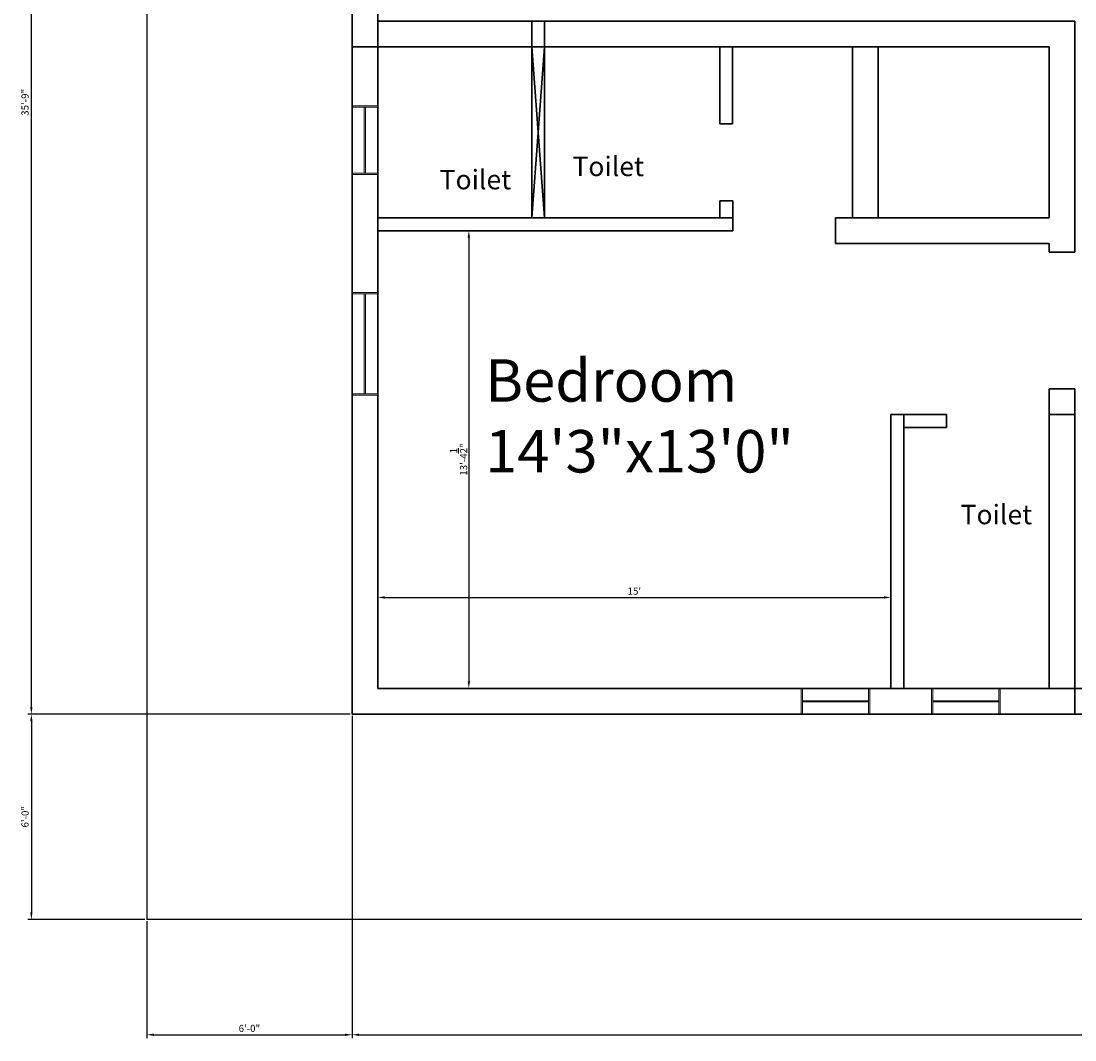
# Model space of a CAD drawing. Units: inches. Extents: x 250205121 to 250208111, y 89832590 to 89833271.
# Tile 10 of 14: x 250207223 to 250207593, y 89832598 to 89832955. Entities that reach past the tile are written whole.
import ezdxf

# ---------------------------------------------------------------- set-up
doc = ezdxf.new("R2010")
doc.units = ezdxf.units.IN
for name, color, linetype, lineweight in [('A-AREA-IDEN', 4, 'Continuous', 18), ('A-WALL', 7, 'Continuous', 35), ('C-PROP', 8, 'Continuous', 25), ('dimensions', 2, 'Continuous', 18), ('window', 4, 'Continuous', 18)]:
    doc.layers.add(name, color=color, linetype=linetype, lineweight=lineweight)
doc.styles.get("Standard").update_dxf_attribs({"font": 'arial.ttf'})
doc.dimstyles.new('ISO-25', dxfattribs={"dimtxt": 2.5, "dimasz": 2.5, "dimexe": 1.25, "dimexo": 0.625, "dimtad": 1, "dimlunit": 4, "dimtxsty": 'Standard', "dimcen": 2.5, "dimadec": 0, "dimazin": 0, "dimtfac": 1, "dimtmove": 0, "dimatfit": 3, "dimfxl": 1, "dimarcsym": 0})

# ---------------------------------------------------------------- blocks, each defined once
blk = doc.blocks.new('*D21')
at = {"layer": 'Defpoints', "color": 0, "transparency": 16777216}
for p in [(250207348.21, 89832771.75), (250207528.21, 89832771.75), (250207528.21, 89832753.11)]:
    blk.add_point(p, dxfattribs=at)
at = {"layer": 'dimensions', "color": 0, "lineweight": -2, "transparency": 16777216}
for p, q in [((250207348.21, 89832771.13), (250207348.21, 89832751.86)), ((250207528.21, 89832771.13), (250207528.21, 89832751.86)), ((250207350.71, 89832753.11), (250207525.71, 89832753.11))]:
    blk.add_line(p, q, dxfattribs=at)
at = {"layer": 'dimensions', "color": 0, "transparency": 16777216}
for points in [[(250207350.71, 89832753.53), (250207350.71, 89832752.7), (250207348.21, 89832753.11)], [(250207525.71, 89832753.53), (250207525.71, 89832752.7), (250207528.21, 89832753.11)]]:
    blk.add_solid(points, dxfattribs=at)
at = {"layer": 'dimensions', "color": 0, "transparency": 16777216, "insert": (250207438.21, 89832755.01), "char_height": 2.5, "attachment_point": 5}
blk.add_mtext("15'", dxfattribs=at)
blk = doc.blocks.new('*D22')
at = {"layer": 'Defpoints', "color": 0, "transparency": 16777216}
for p in [(250207380.17, 89832881.72), (250207380.17, 89832721.22), (250207380.17, 89832721.22)]:
    blk.add_point(p, dxfattribs=at)
at = {"layer": 'dimensions', "color": 0, "lineweight": -2, "transparency": 16777216}
for p, q in [((250207380.17, 89832879.22), (250207380.17, 89832723.72)), ((250207380.8, 89832881.72), (250207381.42, 89832881.72)), ((250207380.8, 89832721.22), (250207381.42, 89832721.22))]:
    blk.add_line(p, q, dxfattribs=at)
at = {"layer": 'dimensions', "color": 0, "transparency": 16777216}
for points in [[(250207379.76, 89832879.22), (250207380.59, 89832879.22), (250207380.17, 89832881.72)], [(250207379.76, 89832723.72), (250207380.59, 89832723.72), (250207380.17, 89832721.22)]]:
    blk.add_solid(points, dxfattribs=at)
at = {"layer": 'dimensions', "color": 0, "transparency": 16777216, "insert": (250207376.6, 89832801.47), "char_height": 2.5, "attachment_point": 5, "rotation": 90}
blk.add_mtext('13\'-4{\\H1x;\\S1/2;}"', dxfattribs=at)
blk = doc.blocks.new('WIN-24IN')
for p, q in [((0, 0), (0, 24.08)), ((0, 24.08), (9, 24.08)), ((0, 23.58), (9, 23.58)), ((4.3, 23.58), (4.3, 0.5)), ((4.7, 23.58), (4.7, 0.5)), ((9, 24.08), (9, 0)), ((9, 0.5), (0, 0.5)), ((9, 0), (0, 0))]:
    blk.add_line(p, q)
blk = doc.blocks.new('WIN-36IN')
for p, q in [((0, 0), (0, 36.08)), ((0, 36.08), (9, 36.08)), ((0, 35.58), (9, 35.58)), ((4.3, 35.58), (4.3, 0.5)), ((4.7, 35.58), (4.7, 0.5)), ((9, 36.08), (9, 0)), ((9, 0.5), (0, 0.5)), ((9, 0), (0, 0))]:
    blk.add_line(p, q)
blk = doc.blocks.new('*D68')
at = {"layer": 'Defpoints', "color": 0, "transparency": 16777216}
for p in [(250207339.21, 89832712.22), (250207267.21, 89832640.22), (250207339.21, 89832599.77)]:
    blk.add_point(p, dxfattribs=at)
at = {"layer": 'dimensions', "color": 0, "lineweight": -2, "transparency": 16777216}
for p, q in [((250207339.21, 89832711.59), (250207339.21, 89832598.52)), ((250207267.21, 89832639.59), (250207267.21, 89832598.52)), ((250207269.71, 89832599.77), (250207336.71, 89832599.77))]:
    blk.add_line(p, q, dxfattribs=at)
at = {"layer": 'dimensions', "color": 0, "transparency": 16777216}
for points in [[(250207269.71, 89832600.18), (250207269.71, 89832599.35), (250207267.21, 89832599.77)], [(250207336.71, 89832600.18), (250207336.71, 89832599.35), (250207339.21, 89832599.77)]]:
    blk.add_solid(points, dxfattribs=at)
at = {"layer": 'dimensions', "color": 0, "transparency": 16777216, "insert": (250207303.21, 89832601.67), "char_height": 2.5, "attachment_point": 5}
blk.add_mtext('6\'-0"', dxfattribs=at)
blk = doc.blocks.new('*D69')
at = {"layer": 'Defpoints', "color": 0, "transparency": 16777216}
for p in [(250207339.21, 89832712.22), (250207226.76, 89832640.22), (250207267.21, 89832640.22)]:
    blk.add_point(p, dxfattribs=at)
at = {"layer": 'dimensions', "color": 0, "lineweight": -2, "transparency": 16777216}
for p, q in [((250207338.58, 89832712.22), (250207225.51, 89832712.22)), ((250207226.76, 89832709.72), (250207226.76, 89832642.72)), ((250207266.58, 89832640.22), (250207225.51, 89832640.22))]:
    blk.add_line(p, q, dxfattribs=at)
at = {"layer": 'dimensions', "color": 0, "transparency": 16777216}
for points in [[(250207226.34, 89832709.72), (250207227.17, 89832709.72), (250207226.76, 89832712.22)], [(250207226.34, 89832642.72), (250207227.17, 89832642.72), (250207226.76, 89832640.22)]]:
    blk.add_solid(points, dxfattribs=at)
at = {"layer": 'dimensions', "color": 0, "transparency": 16777216, "insert": (250207224.86, 89832676.22), "char_height": 2.5, "attachment_point": 5, "rotation": 90}
blk.add_mtext('6\'-0"', dxfattribs=at)
blk = doc.blocks.new('*D70')
at = {"layer": 'Defpoints', "color": 0, "transparency": 16777216}
for p in [(250207339.21, 89832712.22), (250207970.87, 89832712.22), (250207970.87, 89832599.77)]:
    blk.add_point(p, dxfattribs=at)
at = {"layer": 'dimensions', "color": 0, "lineweight": -2, "transparency": 16777216}
for p, q in [((250207339.21, 89832711.59), (250207339.21, 89832598.52)), ((250207970.87, 89832711.59), (250207970.87, 89832598.52)), ((250207341.71, 89832599.77), (250207968.37, 89832599.77))]:
    blk.add_line(p, q, dxfattribs=at)
at = {"layer": 'dimensions', "color": 0, "transparency": 16777216}
for points in [[(250207341.71, 89832600.18), (250207341.71, 89832599.35), (250207339.21, 89832599.77)], [(250207968.37, 89832600.18), (250207968.37, 89832599.35), (250207970.87, 89832599.77)]]:
    blk.add_solid(points, dxfattribs=at)
at = {"layer": 'dimensions', "color": 0, "transparency": 16777216, "insert": (250207655.04, 89832601.68), "char_height": 2.5, "attachment_point": 5}
blk.add_mtext('52\'-7 1/2"', dxfattribs=at)
blk = doc.blocks.new('*D71')
at = {"layer": 'Defpoints', "color": 0, "transparency": 16777216}
for p in [(250207226.76, 89833141.22), (250207339.21, 89833141.22), (250207339.21, 89832712.22)]:
    blk.add_point(p, dxfattribs=at)
at = {"layer": 'dimensions', "color": 0, "lineweight": -2, "transparency": 16777216}
for p, q in [((250207338.58, 89833141.22), (250207225.51, 89833141.22)), ((250207226.76, 89832714.72), (250207226.76, 89833138.72)), ((250207338.58, 89832712.22), (250207225.51, 89832712.22))]:
    blk.add_line(p, q, dxfattribs=at)
at = {"layer": 'dimensions', "color": 0, "transparency": 16777216}
for points in [[(250207226.34, 89833138.72), (250207227.17, 89833138.72), (250207226.76, 89833141.22)], [(250207226.34, 89832714.72), (250207227.17, 89832714.72), (250207226.76, 89832712.22)]]:
    blk.add_solid(points, dxfattribs=at)
at = {"layer": 'dimensions', "color": 0, "transparency": 16777216, "insert": (250207224.85, 89832926.72), "char_height": 2.5, "attachment_point": 5, "rotation": 90}
blk.add_mtext('35\'-9"', dxfattribs=at)

msp = doc.modelspace()

# ---------------------------------------------------------------- linework, layer by layer
at = {"layer": 'A-WALL'}
for p, q in [((250207339.207, 89833089.717), (250207339.207, 89832712.217)), ((250207348.207, 89833089.717), (250207348.207, 89832721.217)), ((250207348.207, 89832955.217), (250207583.707, 89832955.217)), ((250207402.207, 89832955.217), (250207402.207, 89832886.217)), ((250207406.707, 89832955.217), (250207406.707, 89832886.217)), ((250207592.707, 89832955.217), (250207583.707, 89832955.217)), ((250207592.707, 89832946.217), (250207592.707, 89832955.217)), ((250207339.207, 89832946.217), (250207583.707, 89832946.217)), ((250207406.707, 89832946.217), (250207402.207, 89832886.217)), ((250207406.707, 89832886.217), (250207402.207, 89832946.217)), ((250207468.184, 89832919.217), (250207468.184, 89832946.217)), ((250207472.684, 89832946.217), (250207472.684, 89832919.217)), ((250207514.707, 89832946.217), (250207514.707, 89832886.217)), ((250207523.707, 89832946.217), (250207523.707, 89832886.217)), ((250207583.707, 89832946.217), (250207583.707, 89832886.217)), ((250207592.707, 89832946.217), (250207592.707, 89832877.217)), ((250207472.684, 89832919.217), (250207468.184, 89832919.217)), ((250207472.707, 89832892.217), (250207468.207, 89832892.217)), ((250207468.207, 89832892.217), (250207468.207, 89832886.217)), ((250207472.707, 89832886.217), (250207472.707, 89832892.217)), ((250207348.207, 89832886.217), (250207472.707, 89832886.217)), ((250207472.707, 89832886.217), (250207472.707, 89832881.717)), ((250207508.707, 89832886.217), (250207583.707, 89832886.217)), ((250207514.707, 89832886.217), (250207508.707, 89832886.217)), ((250207508.707, 89832886.217), (250207508.707, 89832877.217)), ((250207472.707, 89832881.717), (250207348.207, 89832881.717)), ((250207508.707, 89832877.217), (250207583.707, 89832877.217)), ((250207583.707, 89832877.217), (250207583.707, 89832874.217)), ((250207592.707, 89832877.217), (250207592.707, 89832874.217)), ((250207583.707, 89832874.217), (250207592.707, 89832874.217)), ((250207583.707, 89832826.217), (250207583.707, 89832721.217)), ((250207583.707, 89832826.217), (250207592.707, 89832826.217)), ((250207592.707, 89832826.217), (250207592.707, 89832721.217)), ((250207528.207, 89832799.217), (250207528.207, 89832817.217)), ((250207528.207, 89832817.217), (250207532.707, 89832817.217)), ((250207532.707, 89832799.217), (250207532.707, 89832817.217)), ((250207532.707, 89832817.217), (250207547.707, 89832817.217)), ((250207547.707, 89832817.217), (250207547.707, 89832812.717)), ((250207583.707, 89832799.217), (250207583.707, 89832817.217)), ((250207583.707, 89832817.217), (250207592.707, 89832817.217)), ((250207547.707, 89832812.717), (250207532.707, 89832812.717)), ((250207528.207, 89832721.217), (250207528.207, 89832799.217)), ((250207532.707, 89832721.217), (250207532.707, 89832799.217)), ((250207583.707, 89832739.217), (250207583.707, 89832799.217)), ((250207583.707, 89832721.217), (250207583.707, 89832739.217)), ((250207889.707, 89832721.217), (250207348.207, 89832721.217)), ((250207592.707, 89832721.217), (250207592.707, 89832712.217)), ((250207441.734, 89832712.217), (250207339.207, 89832712.217)), ((250207889.707, 89832712.217), (250207356.707, 89832712.217))]:
    msp.add_line(p, q, dxfattribs=at)
at = {"layer": 'C-PROP'}
for p, q in [((250207267.207, 89833213.217), (250207267.207, 89832640.217)), ((250207592.707, 89832640.217), (250207267.207, 89832640.217)), ((250208069.707, 89832640.217), (250207592.707, 89832640.217))]:
    msp.add_line(p, q, dxfattribs=at)

# ---------------------------------------------------------------- block references
at = {"layer": 'window'}
for name, p in [('WIN-24IN', (250207339.207, 89832901.438)), ('WIN-36IN', (250207339.207, 89832823.996))]:
    msp.add_blockref(name, p, dxfattribs=at)
for p, rotation in [((250207520.79, 89832712.217), 90.00000018666607), ((250207566.468, 89832712.217), 90.00000004712507)]:
    msp.add_blockref('WIN-24IN', p, dxfattribs=dict(at, rotation=rotation))

# ---------------------------------------------------------------- texts
at = {"layer": 'A-AREA-IDEN', "attachment_point": 1}
for s, width, gutter_width, insert, char_height in [('Toilet', 7.46996, 34.11, (250207416.502, 89832907.666), 6.8219), ('Toilet', 7.46996, 34.11, (250207369.933, 89832903.048), 6.8219), ('Bedroom\\P14\'3"x13\'0"', 23.63705, 74.43, (250207385.869, 89832836.626), 14.88606), ('Toilet', 7.46996, 34.11, (250207552.627, 89832785.597), 6.8219)]:
    msp.add_mtext_dynamic_manual_height_columns(s, width=width, gutter_width=gutter_width, heights=[0], dxfattribs=dict(at, insert=insert, char_height=char_height))

# ---------------------------------------------------------------- dimensions: what is measured, and where the dimension line sits
at = {"layer": 'dimensions'}
for base, p1, p2, override, picture, middle in [((250207226.757, 89833141.217), (250207339.207, 89832712.217), (250207339.207, 89833141.217), {"dimdec": 1, "dimlfac": 1, "dimrnd": 0, "dimzin": 1, "dimdsep": 46, "dimlunit": 4, "dimfrac": 2}, '*D71', (250207224.855, 89832926.717)), ((250207380.172, 89832721.217), (250207380.172, 89832881.717), (250207380.172, 89832721.217), {"dimclrd": 0, "dimclre": 0, "dimclrt": 0}, '*D22', (250207376.598, 89832801.467)), ((250207226.757, 89832640.217), (250207339.207, 89832712.217), (250207267.207, 89832640.217), {"dimdec": 1, "dimlfac": 1, "dimrnd": 0, "dimzin": 1, "dimdsep": 46, "dimlunit": 4, "dimfrac": 2}, '*D69', (250207224.856, 89832676.217))]:
    dim = msp.add_linear_dim(base=base, p1=p1, p2=p2, angle=90, dimstyle='ISO-25', override=override, dxfattribs=at)
    dim.commit()
    dim.dimension.update_dxf_attribs({"geometry": picture, "text_midpoint": middle})
for base, p1, p2, override, picture, middle in [((250207528.207, 89832753.112), (250207348.207, 89832771.753), (250207528.207, 89832771.753), {"dimclrd": 0, "dimclre": 0, "dimclrt": 0}, '*D21', (250207438.207, 89832755.014)), ((250207339.207, 89832599.767), (250207267.207, 89832640.217), (250207339.207, 89832712.217), {"dimdec": 1, "dimlfac": 1, "dimrnd": 0, "dimzin": 1, "dimdsep": 46, "dimlunit": 4, "dimfrac": 2}, '*D68', (250207303.207, 89832601.668)), ((250207970.867, 89832599.767), (250207339.207, 89832712.217), (250207970.867, 89832712.217), {"dimdec": 1, "dimlfac": 1, "dimrnd": 0, "dimzin": 1, "dimdsep": 46, "dimlunit": 4, "dimfrac": 2}, '*D70', (250207655.037, 89832601.685))]:
    dim = msp.add_linear_dim(base=base, p1=p1, p2=p2, dimstyle='ISO-25', override=override, dxfattribs=at)
    dim.commit()
    dim.dimension.update_dxf_attribs({"geometry": picture, "text_midpoint": middle})

doc.saveas('drawing.dxf')
